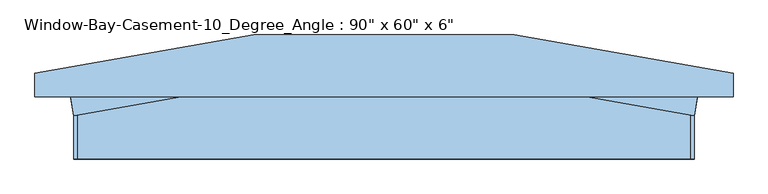
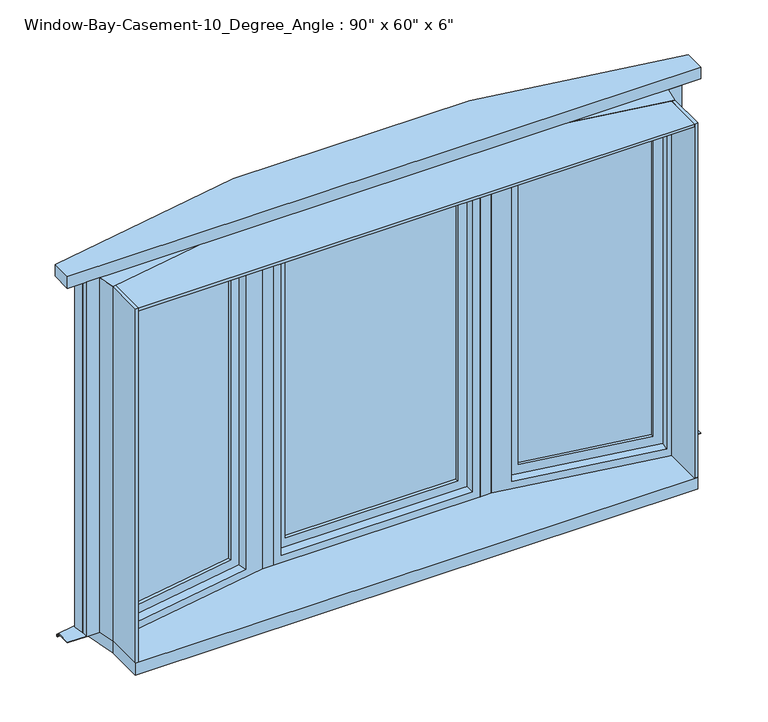
"""IFC4 building model written with IfcOpenShell, lengths in millimetres: window geometry."""

from ifc_helpers import new_model, si_unit, frame, origin, place, context, project, spatial, polyline, outline, extrude, faceted_brep, source, transform, mapped, element, save


def window_bf21e6cb(model_context):
    return source(origin(), model_context, "Body", "SolidModel", [
        extrude(outline(polyline([(1086.3405037, 126.4293252), (1085.2378377, 120.175796), (588.6035631, 207.7458181), (589.7062291, 213.9993474), (1086.3405037, 126.4293252)])), frame((0.0, 0.0, 730.25), z_axis=(0.0, 0.0, 1.0), x_axis=(1.0, 0.0, 0.0)), (0.0, 0.0, 1.0), 1384.3),
        extrude(outline(polyline([(1084.1351718, 113.9222667), (1083.0325059, 107.6687375), (586.3982313, 195.2387597), (587.5008972, 201.4922889), (1084.1351718, 113.9222667)])), frame((0.0, 0.0, 730.25), z_axis=(0.0, 0.0, 1.0), x_axis=(1.0, 0.0, 0.0)), (0.0, 0.0, 1.0), 1384.3),
        extrude(outline(polyline([(1441.45, 57.15), (1441.45, -561.4456588), (-57.15, -561.4456588), (-57.15, 57.15), (1441.45, 57.15)]), holes=[polyline([(1384.3, -504.2956588), (1384.3, 0.0), (0.0, 0.0), (0.0, -504.2956588), (1384.3, -504.2956588)])]), frame((1080.827174, 95.1616791, 730.25), z_axis=(0.17364817766693028, 0.9848077530122081, 0.0), x_axis=(0.0, 0.0, 1.0)), (0.0, 0.0, 1.0), 44.45),
        faceted_brep([(464.7780905, 165.1, 2184.4), (1143.0, 45.5111785, 2184.4), (1155.1293252, 114.3, 2184.4), (1210.6708887, 114.3, 2184.4), (1210.6708887, 136.7463187, 2184.4), (473.6669387, 266.7, 2184.4), (1137.1089371, 85.2376857, 2171.7), (527.9111363, 192.6556946, 2171.7), (538.9377956, 255.1909869, 2171.7), (1148.1355964, 147.772978, 2171.7), (1111.7323538, 51.0245081, 2152.65), (540.0557285, 151.8265214, 2152.65), (546.671724, 189.3476968, 2152.65), (1118.3483494, 88.5456835, 2152.65), (527.9111363, 192.6556946, 673.1), (538.9377956, 255.1909869, 673.1), (540.0557285, 151.8265214, 692.15), (546.671724, 189.3476968, 692.15), (473.6669387, 266.7, 660.4), (1210.6708887, 136.7463187, 660.4), (1210.6708887, 114.3, 660.4), (1155.1293252, 114.3, 660.4), (1143.0, 45.5111785, 660.4), (464.7780905, 165.1, 660.4), (1137.1089371, 85.2376857, 673.1), (1148.1355964, 147.772978, 673.1), (1111.7323538, 51.0245081, 692.15), (1118.3483494, 88.5456835, 692.15)], [[[0, 1, 2, 3, 4, 5]], [[6, 7, 8, 9]], [[10, 11, 12, 13]], [[7, 14, 15, 8]], [[11, 16, 17, 12]], [[18, 19, 20, 21, 22, 23]], [[14, 24, 25, 15]], [[16, 26, 27, 17]], [[22, 21, 2, 1]], [[4, 19, 18, 5], [8, 15, 25, 9]], [[9, 25, 24, 6]], [[6, 24, 14, 7], [12, 17, 27, 13]], [[13, 27, 26, 10]], [[1, 0, 23, 22], [10, 26, 16, 11]], [[5, 18, 23, 0]], [[2, 21, 20, 3]], [[3, 20, 19, 4]]]),
        extrude(outline(polyline([(-1086.3405037, 126.4293252), (-589.7062291, 213.9993474), (-588.6035631, 207.7458181), (-1085.2378377, 120.175796), (-1086.3405037, 126.4293252)])), frame((0.0, 0.0, 730.25), z_axis=(0.0, 0.0, 1.0), x_axis=(1.0, 0.0, 0.0)), (0.0, 0.0, 1.0), 1384.3),
        extrude(outline(polyline([(-1084.1351718, 113.9222667), (-587.5008972, 201.4922889), (-586.3982313, 195.2387597), (-1083.0325059, 107.6687375), (-1084.1351718, 113.9222667)])), frame((0.0, 0.0, 730.25), z_axis=(0.0, 0.0, 1.0), x_axis=(1.0, 0.0, 0.0)), (0.0, 0.0, 1.0), 1384.3),
        extrude(outline(polyline([(1441.45, -57.15), (-57.15, -57.15), (-57.15, 561.4456588), (1441.45, 561.4456588), (1441.45, -57.15)]), holes=[polyline([(1384.3, 504.2956588), (0.0, 504.2956588), (0.0, 0.0), (1384.3, 0.0), (1384.3, 504.2956588)])]), frame((-1080.827174, 95.1616791, 730.25), z_axis=(-0.17364817766693028, 0.9848077530122081, 0.0), x_axis=(0.0, 0.0, 1.0)), (0.0, 0.0, 1.0), 44.45),
        faceted_brep([(-464.7780905, 165.1, 2184.4), (-473.6669387, 266.7, 2184.4), (-1210.6708887, 136.7463187, 2184.4), (-1210.6708887, 114.3, 2184.4), (-1155.1293252, 114.3, 2184.4), (-1143.0, 45.5111785, 2184.4), (-1137.1089371, 85.2376857, 2171.7), (-1148.1355964, 147.772978, 2171.7), (-538.9377956, 255.1909869, 2171.7), (-527.9111363, 192.6556946, 2171.7), (-1111.7323538, 51.0245081, 2152.65), (-1118.3483494, 88.5456835, 2152.65), (-546.671724, 189.3476968, 2152.65), (-540.0557285, 151.8265214, 2152.65), (-538.9377956, 255.1909869, 673.1), (-527.9111363, 192.6556946, 673.1), (-546.671724, 189.3476968, 692.15), (-540.0557285, 151.8265214, 692.15), (-473.6669387, 266.7, 660.4), (-464.7780905, 165.1, 660.4), (-1143.0, 45.5111785, 660.4), (-1155.1293252, 114.3, 660.4), (-1210.6708887, 114.3, 660.4), (-1210.6708887, 136.7463187, 660.4), (-1148.1355964, 147.772978, 673.1), (-1137.1089371, 85.2376857, 673.1), (-1118.3483494, 88.5456835, 692.15), (-1111.7323538, 51.0245081, 692.15)], [[[0, 1, 2, 3, 4, 5]], [[6, 7, 8, 9]], [[10, 11, 12, 13]], [[9, 8, 14, 15]], [[13, 12, 16, 17]], [[18, 19, 20, 21, 22, 23]], [[15, 14, 24, 25]], [[17, 16, 26, 27]], [[20, 5, 4, 21]], [[2, 1, 18, 23], [8, 7, 24, 14]], [[7, 6, 25, 24]], [[6, 9, 15, 25], [12, 11, 26, 16]], [[11, 10, 27, 26]], [[5, 20, 19, 0], [10, 13, 17, 27]], [[1, 0, 19, 18]], [[4, 3, 22, 21]], [[3, 2, 23, 22]]]),
        faceted_brep([(-478.1113628, 317.5, 660.4), (-478.1113628, 317.5, 653.0697935), (478.1113628, 317.5, 653.0697935), (478.1113628, 317.5, 660.4), (-473.6669387, 266.7, 663.1486341), (-473.6669387, 266.7, 660.4), (473.6669387, 266.7, 660.4), (473.6669387, 266.7, 663.1486341), (-478.2335845, 318.897, 654.4483503), (-478.2335845, 318.897, 663.1486341), (478.2335845, 318.897, 663.1486341), (478.2335845, 318.897, 654.4483503), (479.3446905, 331.597, 652.2089977), (-479.3446905, 331.597, 652.2089977), (479.3446905, 331.597, 643.2668038), (-479.3446905, 331.597, 643.2668038), (-478.9980255, 327.6346, 644.7270038), (-478.9980255, 327.6346, 643.2668038), (478.9980255, 327.6346, 643.2668038), (478.9980255, 327.6346, 644.7270038), (-479.2046912, 329.9968, 650.8662705), (-479.2046912, 329.9968, 644.7270038), (479.2046912, 329.9968, 644.7270038), (479.2046912, 329.9968, 650.8662705), (-1286.8726318, 174.8935673, 660.4), (-1286.8726318, 174.8935673, 653.0697935), (1286.8726318, 174.8935673, 660.4), (1286.8726318, 114.3, 660.4), (1210.6726318, 114.3, 660.4), (1210.6726318, 136.7460114, 660.4), (-1210.6726318, 136.7460114, 660.4), (-1210.6726318, 114.3, 660.4), (-1286.8726318, 114.3, 660.4), (-1210.6726318, 136.7460114, 663.1486341), (1210.6726318, 136.7460114, 663.1486341), (1210.6726318, 114.3, 663.1486341), (1286.8726318, 114.3, 663.1486341), (1286.8726318, 176.3121183, 663.1486341), (-1286.8726318, 176.3121183, 663.1486341), (-1286.8726318, 114.3, 663.1486341), (-1210.6726318, 114.3, 663.1486341), (-1286.8726318, 176.3121183, 654.4483503), (-1286.8726318, 189.2080363, 652.2089977), (-1286.8726318, 189.2080363, 643.2668038), (1286.8726318, 189.2080363, 643.2668038), (1286.8726318, 185.1845099, 643.2668038), (-1286.8726318, 185.1845099, 643.2668038), (-1286.8726318, 185.1845099, 644.7270038), (1286.8726318, 185.1845099, 644.7270038), (1286.8726318, 187.5831506, 644.7270038), (-1286.8726318, 187.5831506, 644.7270038), (-1286.8726318, 187.5831506, 650.8662705), (1286.8726318, 174.8935673, 653.0697935), (1286.8726318, 176.3121183, 654.4483503), (1286.8726318, 189.2080363, 652.2089977), (1286.8726318, 187.5831506, 650.8662705)], [[[0, 1, 2, 3]], [[4, 5, 6, 7]], [[8, 9, 10, 11]], [[8, 11, 12, 13]], [[13, 12, 14, 15]], [[16, 17, 18, 19]], [[20, 21, 22, 23]], [[2, 1, 20, 23]], [[1, 0, 24, 25]], [[0, 3, 26, 27, 28, 29, 6, 5, 30, 31, 32, 24]], [[5, 4, 33, 30]], [[4, 7, 34, 35, 36, 37, 10, 9, 38, 39, 40, 33]], [[9, 8, 41, 38]], [[8, 13, 42, 41]], [[13, 15, 43, 42]], [[15, 14, 44, 45, 18, 17, 46, 43]], [[17, 16, 47, 46]], [[16, 19, 48, 49, 22, 21, 50, 47]], [[21, 20, 51, 50]], [[20, 1, 25, 51]], [[3, 2, 52, 26]], [[7, 6, 29, 34]], [[11, 10, 37, 53]], [[12, 11, 53, 54]], [[14, 12, 54, 44]], [[19, 18, 45, 48]], [[23, 22, 49, 55]], [[2, 23, 55, 52]], [[25, 24, 32, 39, 38, 41, 42, 43, 46, 47, 50, 51]], [[27, 26, 52, 55, 49, 48, 45, 44, 54, 53, 37, 36]], [[33, 40, 31, 30]], [[40, 39, 32, 31]], [[36, 35, 28, 27]], [[35, 34, 29, 28]]]),
        extrude(outline(polyline([(-1179.4049856, 142.259341), (-1210.6726318, 136.7460114), (-1218.3912933, 180.520716), (-1187.1236471, 186.0340456), (-1179.4049856, 142.259341)])), frame((0.0, 0.0, 663.1486341), z_axis=(0.0, 0.0, 1.0), x_axis=(1.0, 0.0, 0.0)), (0.0, 0.0, 1.0), 1521.2513659),
        extrude(outline(polyline([(1179.4049856, 142.259341), (1187.1236471, 186.0340456), (1218.3912933, 180.520716), (1210.6726318, 136.7460114), (1179.4049856, 142.259341)])), frame((0.0, 0.0, 663.1486341), z_axis=(0.0, 0.0, 1.0), x_axis=(1.0, 0.0, 0.0)), (0.0, 0.0, 1.0), 1521.2513659),
        extrude(outline(polyline([(480.3335749, 342.9), (1286.8726318, 200.6854033), (1286.8726318, 114.3), (-1286.8708887, 114.3), (-1286.8708887, 200.6857106), (-480.3335749, 342.9), (480.3335749, 342.9)])), frame((0.0, 0.0, 2184.4), z_axis=(0.0, 0.0, 1.0), x_axis=(1.0, 0.0, 0.0)), (0.0, 0.0, 1.0), 50.8),
        extrude(outline(polyline([(-420.0891737, 266.7), (-420.0891737, 165.1), (-464.7780905, 165.1), (-473.6669387, 266.7), (-420.0891737, 266.7)])), frame((0.0, 0.0, 660.4), z_axis=(0.0, 0.0, 1.0), x_axis=(1.0, 0.0, 0.0)), (0.0, 0.0, 1.0), 1524.0),
        extrude(outline(polyline([(473.6669387, 266.7), (464.7780905, 165.1), (420.0891737, 165.1), (420.0891737, 266.7), (473.6669387, 266.7)])), frame((0.0, 0.0, 660.4), z_axis=(0.0, 0.0, 1.0), x_axis=(1.0, 0.0, 0.0)), (0.0, 0.0, 1.0), 1524.0),
        faceted_brep([(407.3891737, 203.2, 673.1), (407.3891737, 266.7, 673.1), (-407.3891737, 266.7, 673.1), (-407.3891737, 203.2, 673.1), (388.3391737, 165.1, 692.15), (388.3391737, 203.2, 692.15), (-388.3391737, 203.2, 692.15), (-388.3391737, 165.1, 692.15), (420.0891737, 266.7, 660.4), (420.0891737, 165.1, 660.4), (-420.0891737, 165.1, 660.4), (-420.0891737, 266.7, 660.4), (-407.3891737, 266.7, 2171.7), (-407.3891737, 203.2, 2171.7), (-388.3391737, 203.2, 2152.65), (-388.3391737, 165.1, 2152.65), (-420.0891737, 165.1, 2184.4), (-420.0891737, 266.7, 2184.4), (407.3891737, 266.7, 2171.7), (407.3891737, 203.2, 2171.7), (388.3391737, 203.2, 2152.65), (388.3391737, 165.1, 2152.65), (420.0891737, 165.1, 2184.4), (420.0891737, 266.7, 2184.4)], [[[0, 1, 2, 3]], [[4, 5, 6, 7]], [[8, 9, 10, 11]], [[3, 2, 12, 13]], [[7, 6, 14, 15]], [[11, 10, 16, 17]], [[13, 12, 18, 19]], [[15, 14, 20, 21]], [[17, 16, 22, 23]], [[11, 17, 23, 8], [1, 18, 12, 2]], [[19, 18, 1, 0]], [[3, 13, 19, 0], [5, 20, 14, 6]], [[21, 20, 5, 4]], [[9, 22, 16, 10], [7, 15, 21, 4]], [[23, 22, 9, 8]]]),
        extrude(outline(polyline([(350.2391737, 234.95), (350.2391737, 228.6), (-350.2391737, 228.6), (-350.2391737, 234.95), (350.2391737, 234.95)])), frame((0.0, 0.0, 730.25), z_axis=(0.0, 0.0, 1.0), x_axis=(1.0, 0.0, 0.0)), (0.0, 0.0, 1.0), 1384.3),
        extrude(outline(polyline([(350.2391737, 222.25), (350.2391737, 215.9), (-350.2391737, 215.9), (-350.2391737, 222.25), (350.2391737, 222.25)])), frame((0.0, 0.0, 730.25), z_axis=(0.0, 0.0, 1.0), x_axis=(1.0, 0.0, 0.0)), (0.0, 0.0, 1.0), 1384.3),
        extrude(outline(polyline([(1143.0, -114.3), (-1143.0, -114.3), (-1143.0, 45.5111785), (-1169.4639823, 195.59588), (-478.1113628, 317.5), (478.1113628, 317.5), (1169.4639823, 195.59588), (1143.0, 45.5111785), (1143.0, -114.3)])), frame((0.0, 0.0, 609.6), z_axis=(0.0, 0.0, 1.0), x_axis=(1.0, 0.0, 0.0)), (0.0, 0.0, 1.0), 50.8),
        extrude(outline(polyline([(2171.7, -407.3891737), (673.1, -407.3891737), (673.1, 407.3891737), (2171.7, 407.3891737), (2171.7, -407.3891737)]), holes=[polyline([(2114.55, 350.2391737), (730.25, 350.2391737), (730.25, -350.2391737), (2114.55, -350.2391737), (2114.55, 350.2391737)])]), frame((0.0, 203.2, 0.0), z_axis=(0.0, 1.0, 0.0), x_axis=(0.0, 0.0, 1.0)), (0.0, 0.0, 1.0), 44.45),
        extrude(outline(polyline([(-1143.0, -114.3), (-1143.0, 45.5111785), (-1130.3, 47.7505311), (-1130.3, -114.3), (-1143.0, -114.3)])), frame((0.0, 0.0, 660.4), z_axis=(0.0, 0.0, 1.0), x_axis=(1.0, 0.0, 0.0)), (0.0, 0.0, 1.0), 1524.0),
        extrude(outline(polyline([(1143.0, -114.3), (1130.3, -114.3), (1130.3, 47.7505311), (1143.0, 45.5111785), (1143.0, -114.3)])), frame((0.0, 0.0, 660.4), z_axis=(0.0, 0.0, 1.0), x_axis=(1.0, 0.0, 0.0)), (0.0, 0.0, 1.0), 1524.0),
        extrude(outline(polyline([(-464.7780905, 165.1), (464.7780905, 165.1), (1130.3, 47.7505311), (1130.3, -114.3), (-1130.3, -114.3), (-1130.3, 47.7505311), (-464.7780905, 165.1)])), frame((0.0, 0.0, 2171.7), z_axis=(0.0, 0.0, 1.0), x_axis=(1.0, 0.0, 0.0)), (0.0, 0.0, 1.0), 12.7),
    ])


if __name__ == "__main__":
    model = new_model("IFC4")
    model_context = context("Model", 3, world=origin())
    ifc_project = project(units=[si_unit("LENGTHUNIT", "METRE", prefix="MILLI")], contexts=[model_context])
    site = spatial("IfcSite", under=ifc_project)
    building = spatial("IfcBuilding", under=site)
    placement = place(None, origin())
    window_shape = window_bf21e6cb(model_context)
    element("IfcWindow", 1, ObjectType="Window-Bay-Casement-10_Degree_Angle : 90\" x 60\" x 6\"", at=placement, inside=building, context=model_context, shape_type="MappedRepresentation", body=[
        mapped(window_shape, transform((0.0, 0.0, 0.0), x_axis=(1.0, 0.0, 0.0), y_axis=(0.0, 1.0, 0.0), z_axis=(0.0, 0.0, 1.0))),
    ])
    save(model, "model.ifc")

# Revit data of these elements
# Type "Window-Bay-Casement-10_Degree_Angle : 90\" x 60\" x 6\""
#   Type Mark = "18"
#   Fire Rating = "0.5h"
#   Assembly Code = "B2020100"
#   Analytic Construction = "Double glazing - domestic"
#   Width of Middle Sash = 2' - 9.07789"
#   Width = 7' - 6"
#   Visual Light Transmittance = 0.81
#   Thermal Resistance (R) = 1.8146 (h·ft²·°F)/BTU
#   Solar Heat Gain Coefficient = 0.76
#   Rough Width = 7' - 6 1/2"
#   Rough Height = 5' - 0 1/2"
#   Length 4 = 0' - 0.24059"
#   Length 3 = 0' - 0 7/64"
#   Length 2 = 3' - 1.29661"
#   Length 1 = 2' - 2.46106"
#   Wall Thickness [instance default] = 0' - 6"
#   Trim Width = 7' - 10.21872"
#   Trim Height = 5' - 0"
#   Height 1 = 5' - 2"
#   Height = 5' - 0"
#   Heat Transfer Coefficient (U) = 0.5511 BTU/(h·ft²·°F)
#   Depth = 0' - 6"
#   Default Sill Height = 2' - 0"
#   Angle 1 = 5.00°
#   Angle = 10.00°
#   Center Muntin Visibility = yes
#   Side Muntin Visibility = yes
#   Interior Trim Visibility [instance default] = yes
#   Exterior Trim Visibility [instance default] = yes
#   Center Muntin Pattern = Muntin Pattern_2x2 : Muntin Pattern_2x2
#   Side Muntin Pattern = Muntin Pattern_2x2 : Muntin Pattern_2x2
#   Interior Trim Material = Wood - Stained
#   Exterior Trim Material = Clad - White
#   Exterior Trim = element 406593
#   Interior Trim = Trim-Window-Interior-Flat : Picture Frame
#   Interior Frame Material = Wood - Stained
#   Glass Panel Material = Glass
#   Exterior Frame Material = Clad - White
#   Wall Closure = (empty or 0)
# Element 1 (IfcWindow, "Window-Bay-Casement-10_Degree_Angle : 90\" x 60\" x 6\"")
#   Wall Thickness = 0' - 9"
#   Materials on its faces: "Clad - White", "Wood - Stained", "Glass"
# Materials
#   "Wood - Stained": class "Wood", colour RGB 224 178 126, transparency 0, Cost = 0
#   "Clad - White": class "Wood", colour RGB 242 242 238, transparency 0, Cost = 0
#   "Glass": class "Glass", colour RGB 0 128 192, transparency 0.75, Description = "Soda Lime Glass", Cost = 0
